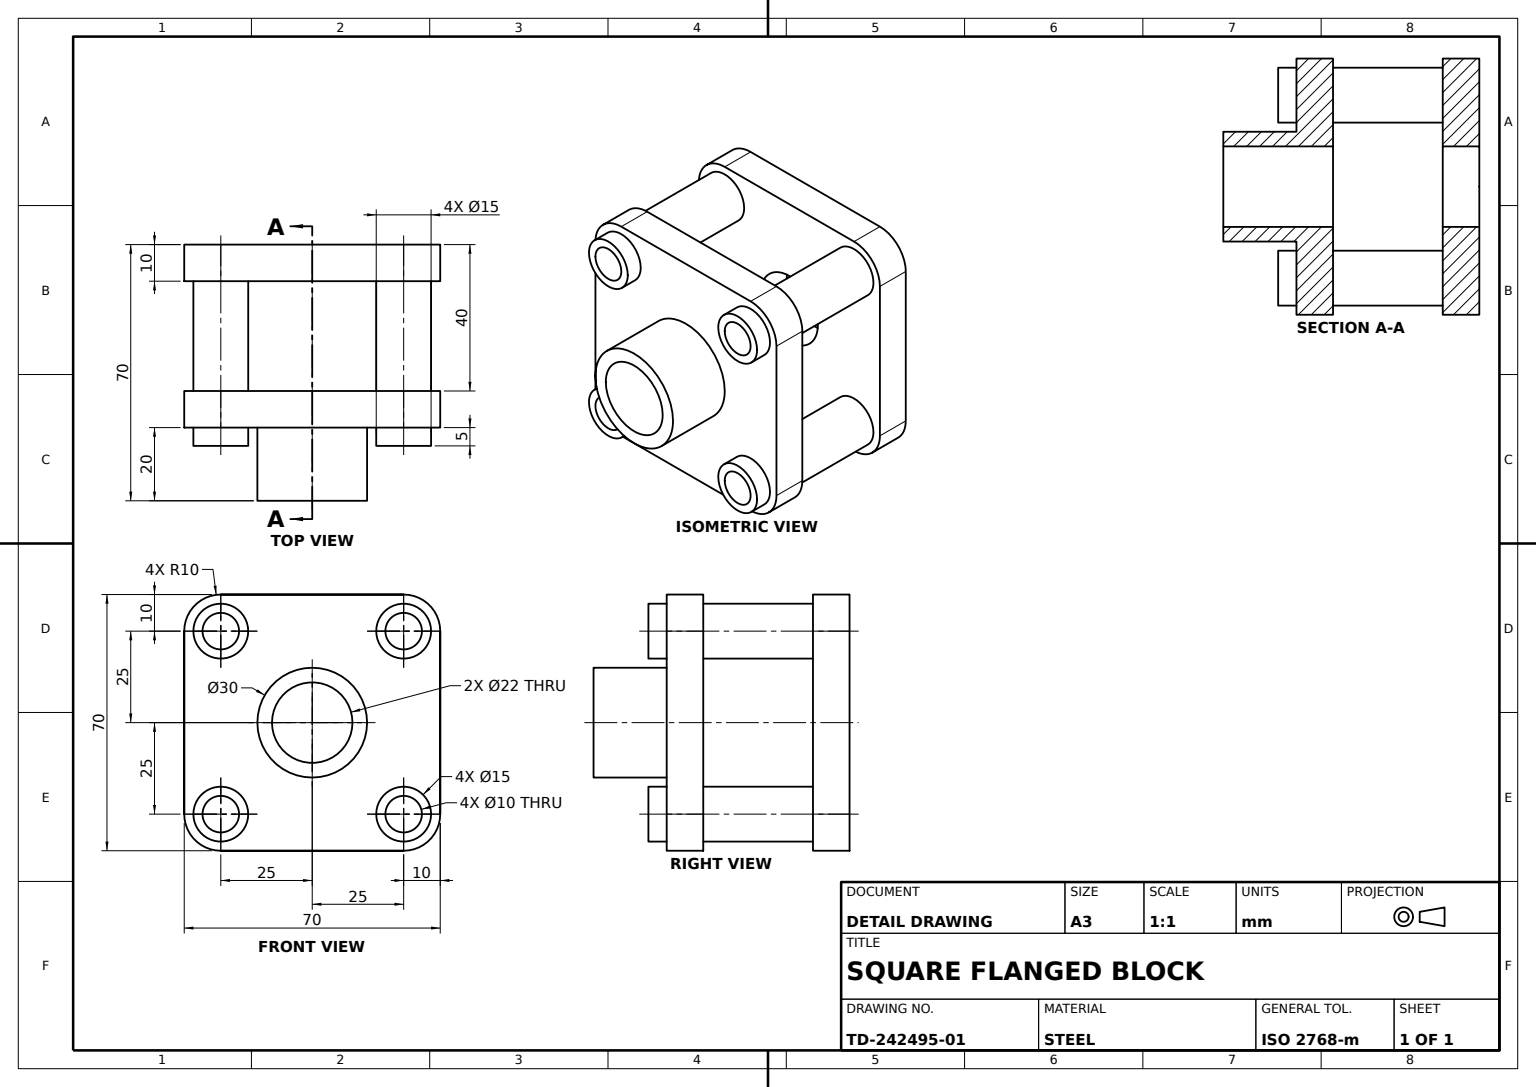
from build123d import *

# Parameters (mm, degrees)
BASE_PLATE_SKETCH_W             = 70
BASE_PLATE_SKETCH_H             = 70
BASE_PLATE_DEPTH                = 10
CORNER_POSTS_SKETCH_R           = 7.5
CORNER_POSTS_4X_DEPTH           = 30
TOP_PLATE_SKETCH_W              = 70
TOP_PLATE_SKETCH_H              = 70
TOP_PLATE_DEPTH                 = 10
POST_BOSSES_SKETCH_R            = 7.5
POST_BOSSES_SKETCH_R_2          = 5
POST_BOSSES_4X_DEPTH            = 5
CENTRE_BOSS_SKETCH_R            = 15
CENTRE_BOSS_SKETCH_R_2          = 11
CENTRE_BOSS_30_DEPTH            = 20
CENTRE_BORE_SKETCH_R            = 11
CENTRE_BORE_CUT_DEPTH           = 111.905365064
POST_HOLES_SKETCH_R             = 5
POST_HOLES_4X_DEPTH             = 111.905365064
TOP_PLATE_CORNER_FILLETS_R10_R  = 10
BASE_PLATE_CORNER_FILLETS_R10_R = 10


with BuildPart() as part:
    # Base Plate Sketch → Base Plate (new body)
    with BuildSketch(Plane.XY):
        with Locations((35, 35)):
            Rectangle(BASE_PLATE_SKETCH_W, BASE_PLATE_SKETCH_H)
    extrude(amount=BASE_PLATE_DEPTH)

    # Corner Posts Sketch → Corner Posts 4x (add)
    with BuildSketch(Plane.XY.offset(10)):
        with Locations((10, 10)):
            Circle(CORNER_POSTS_SKETCH_R)
        with Locations((60, 10)):
            Circle(CORNER_POSTS_SKETCH_R)
        with Locations((60, 60)):
            Circle(CORNER_POSTS_SKETCH_R)
        with Locations((10, 60)):
            Circle(CORNER_POSTS_SKETCH_R)
    extrude(amount=CORNER_POSTS_4X_DEPTH)

    # Top Plate Sketch → Top Plate (add)
    with BuildSketch(Plane.XY.offset(40)):
        with Locations((35, 35)):
            Rectangle(TOP_PLATE_SKETCH_W, TOP_PLATE_SKETCH_H)
    extrude(amount=TOP_PLATE_DEPTH)

    # Post Bosses Sketch → Post Bosses 4x (add)
    # profile 1 of 4: a face of its own
    with BuildSketch(Plane.XY.offset(50)):
        with Locations((10, 60)):
            Circle(POST_BOSSES_SKETCH_R)
        with Locations((10, 60)):
            Circle(POST_BOSSES_SKETCH_R_2, mode=Mode.SUBTRACT)
    # profile 2 of 4: a face of its own
    with BuildSketch(Plane.XY.offset(50)):
        with Locations((60, 60)):
            Circle(POST_BOSSES_SKETCH_R)
        with Locations((60, 60)):
            Circle(POST_BOSSES_SKETCH_R_2, mode=Mode.SUBTRACT)
    # profile 3 of 4: a face of its own
    with BuildSketch(Plane.XY.offset(50)):
        with Locations((10, 10)):
            Circle(POST_BOSSES_SKETCH_R)
        with Locations((10, 10)):
            Circle(POST_BOSSES_SKETCH_R_2, mode=Mode.SUBTRACT)
    # profile 4 of 4: a face of its own
    with BuildSketch(Plane.XY.offset(50)):
        with Locations((60, 10)):
            Circle(POST_BOSSES_SKETCH_R)
        with Locations((60, 10)):
            Circle(POST_BOSSES_SKETCH_R_2, mode=Mode.SUBTRACT)
    extrude(amount=POST_BOSSES_4X_DEPTH)

    # Centre Boss Sketch → Centre Boss Ø30 (add)
    with BuildSketch(Plane.XY.offset(50)):
        with Locations(Location((35, 35, 0), (0, 0, 180))):
            Circle(CENTRE_BOSS_SKETCH_R)
        with Locations((35, 35)):
            Circle(CENTRE_BOSS_SKETCH_R_2, mode=Mode.SUBTRACT)
    extrude(amount=CENTRE_BOSS_30_DEPTH)

    # Centre Bore Sketch → Centre Bore Cut (cut, through all)
    with BuildSketch(Plane.XY.offset(50)):
        with Locations(Location((35, 35, 0), (0, 0, 180))):
            Circle(CENTRE_BORE_SKETCH_R)
    extrude(amount=-CENTRE_BORE_CUT_DEPTH, mode=Mode.SUBTRACT)

    # Post Holes Sketch → Post Holes 4x (cut, through all)
    with BuildSketch(Plane.XY.offset(50)):
        with Locations((60, 60)):
            Circle(POST_HOLES_SKETCH_R)
        with Locations((10, 60)):
            Circle(POST_HOLES_SKETCH_R)
        with Locations((60, 10)):
            Circle(POST_HOLES_SKETCH_R)
        with Locations((10, 10)):
            Circle(POST_HOLES_SKETCH_R)
    extrude(amount=-POST_HOLES_4X_DEPTH, mode=Mode.SUBTRACT)

    # Top Plate Corner Fillets R10
    top_plate_corner_fillets_r10_edges = [part.edges().sort_by_distance(p)[0] for p in [
        (0, 70, 45),
        (0, 0, 45),
        (70, 0, 45),
        (70, 70, 45),
    ]]
    fillet(top_plate_corner_fillets_r10_edges, radius=TOP_PLATE_CORNER_FILLETS_R10_R)

    # Base Plate Corner Fillets R10
    base_plate_corner_fillets_r10_edges = [part.edges().sort_by_distance(p)[0] for p in [
        (0, 70, 5),
        (70, 70, 5),
        (70, 0, 5),
        (0, 0, 5),
    ]]
    fillet(base_plate_corner_fillets_r10_edges, radius=BASE_PLATE_CORNER_FILLETS_R10_R)


solid = part.part
